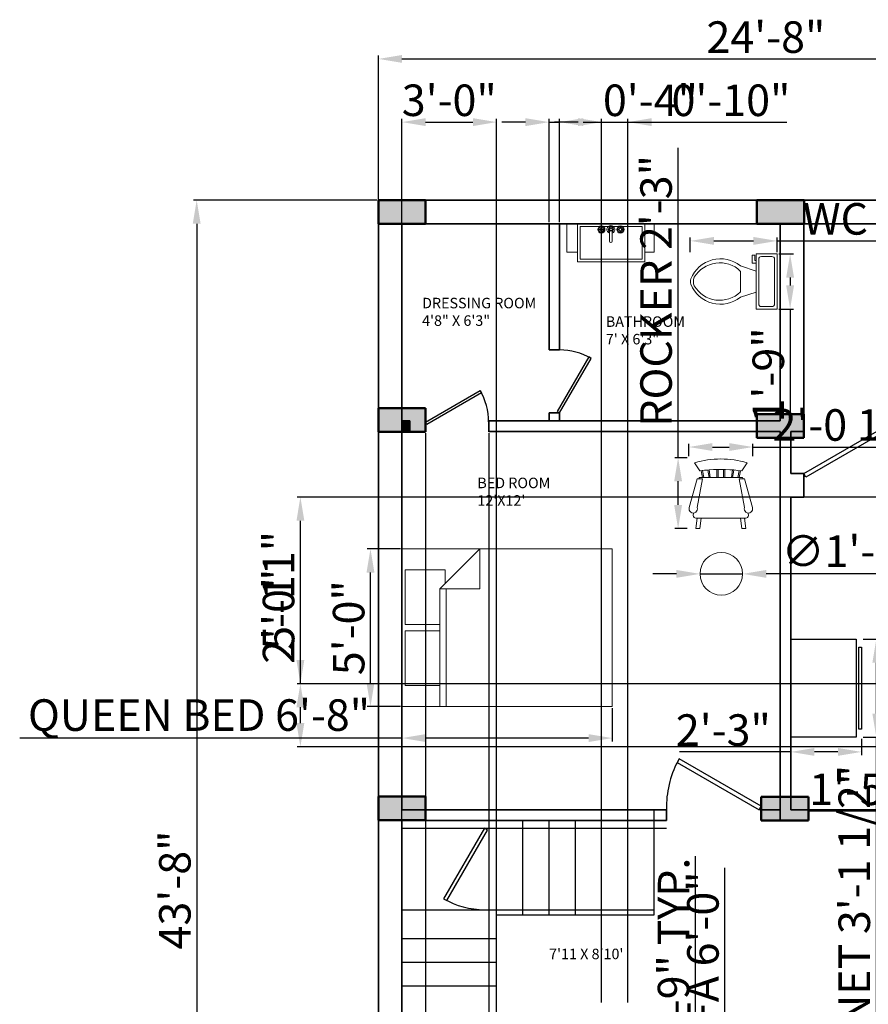
# Model space of a CAD drawing. Units: inches. Extents: x 1132 to 1713, y 3115 to 3781.
# Tile 2 of 4: x 1132 to 1455, y 3365 to 3740. Entities that reach past the tile are written whole.
import ezdxf

# ---------------------------------------------------------------- set-up
doc = ezdxf.new("R2010")
doc.units = ezdxf.units.IN
for name, color, linetype, lineweight in [('A-ANNO-DIMS', 2, 'Continuous', 18), ('A-AREA-IDEN', 7, 'Continuous', 18), ('A-COLS', 1, 'Continuous', 50), ('A-COLS-PATT', 252, 'Continuous', 13), ('A-DOOR', 3, 'Continuous', 25), ('A-FLOR-CASE', 30, 'Continuous', 25), ('A-FLOR-FIXT', 9, 'Continuous', 18), ('A-FLOR-STRS', 7, 'Continuous', 25), ('A-FURN', 8, 'Continuous', 18), ('A-WALL', 7, 'Continuous', 35)]:
    doc.layers.add(name, color=color, linetype=linetype, lineweight=lineweight)
doc.styles.get("Standard").update_dxf_attribs({"font": 'arial.ttf'})
doc.dimstyles.new('ISO-25', dxfattribs={"dimtxt": 12, "dimasz": 9, "dimexe": 1.25, "dimexo": 0.625, "dimtad": 1, "dimdec": 0, "dimrnd": 2, "dimlunit": 3, "dimtxsty": 'Standard', "dimcen": 2.5, "dimadec": 0, "dimazin": 0, "dimtfac": 1, "dimtdec": 0, "dimtmove": 0, "dimatfit": 3, "dimfxl": 1, "dimarcsym": 0})

# ---------------------------------------------------------------- blocks, each defined once
blk = doc.blocks.new('*U2')
for p, q in [((0, 0), (0, -6)), ((40, 0), (40, -6))]:
    blk.add_line(p, q)
blk.add_lwpolyline([(0, 0), (34.64, 20), (35.52, 18.48), (0.87, -1.52)], close=True)
blk.add_arc((0, 0), 40, 0, 30)
blk = doc.blocks.new('*U4')
for p, q in [((0, 0), (0, -6)), ((-40, 0), (-40, -6))]:
    blk.add_line(p, q)
blk.add_lwpolyline([(0, 0), (-34.64, 20), (-35.52, 18.48), (-0.88, -1.52)], close=True)
blk.add_arc((0, 0), 40, 150, 180)
blk = doc.blocks.new('*U3')
for p, q in [((0, 0), (0, 6)), ((40, 0), (40, 6))]:
    blk.add_line(p, q)
blk.add_lwpolyline([(0, 0), (34.64, -20), (35.52, -18.48), (0.87, 1.52)], close=True)
blk.add_arc((0, 0), 40, 330, 0)
blk = doc.blocks.new('*U5')
for p, q in [((0, 0), (0, -6)), ((-40, 0), (-40, -6))]:
    blk.add_line(p, q)
blk.add_lwpolyline([(0, 0), (-34.64, 20), (-35.52, 18.48), (-0.88, -1.52)], close=True)
blk.add_arc((0, 0), 40, 150, 180)
blk = doc.blocks.new('Toilet - top')
for p, q in [((9.5, -6), (9.5, -2)), ((-10, -8.5), (-8, -8.5)), ((-10, -9.5), (-10, -8.5)), ((-7, -9.5), (-10, -9.5)), ((-8, -8.5), (-8, -8)), ((-7, -8), (-7, -9.5)), ((-4, -8), (-6, -14)), ((4, -8), (6, -14)), ((4, -14), (-4, -14))]:
    blk.add_line(p, q)
blk.add_lwpolyline([(10.5, -8), (10.5, 0), (-10.5, 0), (-10.5, -8)], close=True)
for points in [[(-9.5, -2), (-9.5, -6)], [(8.5, -1), (-8.5, -1)], [(-8.5, -7), (8.5, -7)]]:
    blk.add_lwpolyline(points)
for centre, radius, start, end in [((-8.62, -1.88), 0.884, 81.8699, 188.1301), ((8.62, -1.88), 0.884, 351.8699, 98.1301), ((-8.62, -6.12), 0.884, 171.8699, 278.1301), ((8.62, -6.12), 0.884, 261.8699, 8.1301), ((3.52, -21.58), 12.17, 141.4691, 247.9714), ((4.2, -21.82), 11.33, 136.3677, 238.9468), ((-3.52, -21.58), 12.17, 292.0284, 38.5307), ((-4.2, -21.82), 11.33, 301.053, 43.6321), ((0, -27.88), 4, 245.7318, 294.2682), ((0, -29), 4, 254.8605, 285.1395)]:
    blk.add_arc(centre, radius, start, end)
blk = doc.blocks.new('Bed - Queen')
for p, q in [((0, -80.00003), (0, 0)), ((0, 0), (59.99999, 0)), ((59.99999, 0), (59.99999, -80.00003)), ((7.99999, -1.2), (28.79998, -1.2)), ((7.99999, -14.4), (7.99999, -1.2)), ((28.79998, -1.2), (28.79998, -14.4)), ((31.19999, -1.2), (51.99999, -1.2)), ((31.19999, -14.4), (31.19999, -1.2)), ((51.99999, -1.2), (51.99999, -16.4)), ((0, -14.4), (44.8, -14.4)), ((59.99999, -29.6), (44.8, -14.4)), ((44.8, -14.4), (44.8, -29.6)), ((44.8, -16.8), (0, -16.8)), ((51.99999, -16.4), (46.79936, -16.4)), ((44.8, -29.6), (59.99999, -29.6)), ((59.99999, -80.00003), (0, -80.00003))]:
    blk.add_line(p, q)
blk = doc.blocks.new('Chair - Rocking')
for p, q in [((-8, -4.5), (-10, -1.5)), ((8, -4.5), (10, -1.5)), ((-8.23428, -6.99939), (-8.3093, -7.47958)), ((-8.23041, -7), (8.23915, -7)), ((-7.5, -4.5), (-7, -7)), ((-6.5, -7), (-7.02225, -4.43)), ((-4.5, -7), (-4.96674, -4.19951)), ((-4, -7), (-4.40532, -4.16272)), ((-1.5, -4.05012), (-1.5, -7)), ((-1, -7), (-1, -4.05012)), ((1, -7), (1, -4.04655)), ((1.5, -4.05012), (1.5, -7)), ((4, -7), (4.40187, -4.18694)), ((4.5, -7), (4.96761, -4.19437)), ((6.5, -7), (7, -4.4057)), ((7.5, -4.5), (7, -7)), ((8.31071, -7.48854), (8.23449, -7.00073)), ((-9, -7.5), (-12, -18.49999)), ((-7, -7.5), (-9, -7.5)), ((-9, -18.49999), (-7, -7.5)), ((7, -7.5), (9, -7.5)), ((9, -18.49999), (7, -7.5)), ((9, -7.5), (12, -18.49999)), ((-10.36644, -20.64523), (-10.5, -21.49999)), ((10.5, -21.49999), (10.3575, -20.58798)), ((-9, -22.49999), (-9.5, -26.49999)), ((0, -22.49999), (-9.5, -22.49999)), ((-8, -26.49999), (-7.5, -22.49999)), ((0, -22.49999), (9.5, -22.49999)), ((8, -26.49999), (7.5, -22.49999)), ((9, -22.49999), (9.5, -26.49999)), ((-9.5, -26.49999), (-8, -26.49999)), ((9.5, -26.49999), (8, -26.49999))]:
    blk.add_line(p, q)
for centre, radius, start, end in [((0, -34.08333), 34.08333, 72.93847, 107.0615), ((0, -68.25004), 64.25, 93.92211, 97.15267), ((0, -68.25004), 64.25, 82.84733, 93.92211), ((-10.5, -18.99999), 1.58114, 161.5651, 18.43495), ((10.5, -18.99999), 1.58114, 161.5651, 18.43495), ((-9.5, -21.49999), 1, 180, 270), ((9.5, -21.49999), 1, 270, 0)]:
    blk.add_arc(centre, radius, start, end)
blk = doc.blocks.new('Wall Cabinet - 18 x 12 in side')
for points in [[(-12, -18), (-12, 0), (0, 0), (0, -18)], [(-13, -16.5), (-13, -1.5), (-12.5, -1.5), (-12.5, -16.5)]]:
    blk.add_lwpolyline(points, close=True)
blk = doc.blocks.new('*D18')
at = {"layer": 'A-ANNO-DIMS', "color": 0, "lineweight": -2, "transparency": 16777216}
for p, q in [((1267.53, 3670.88), (1197.76, 3670.88)), ((1199.01, 3661.88), (1199.01, 3154.88)), ((1267.53, 3145.88), (1197.76, 3145.88))]:
    blk.add_line(p, q, dxfattribs=at)
at = {"layer": 'A-ANNO-DIMS', "color": 0, "transparency": 16777216}
for points in [[(1197.51, 3661.88), (1200.51, 3661.88), (1199.01, 3670.88)], [(1197.51, 3154.88), (1200.51, 3154.88), (1199.01, 3145.88)]]:
    blk.add_solid(points, dxfattribs=at)
at = {"layer": 'Defpoints', "color": 0, "transparency": 16777216}
for p in [(1268.16, 3670.88), (1199.01, 3145.88), (1268.16, 3145.88)]:
    blk.add_point(p, dxfattribs=at)
at = {"layer": 'A-ANNO-DIMS', "color": 0, "transparency": 16777216, "insert": (1192.25, 3408.38), "char_height": 12, "attachment_point": 5, "rotation": 90}
blk.add_mtext('43\'-8"', dxfattribs=at)
blk = doc.blocks.new('*D19')
at = {"layer": 'A-ANNO-DIMS', "color": 0, "lineweight": -2, "transparency": 16777216}
for p, q in [((1268.16, 3667), (1268.16, 3725.86)), ((1277.16, 3724.61), (1554.22, 3724.61)), ((1563.22, 3671.51), (1563.22, 3725.86))]:
    blk.add_line(p, q, dxfattribs=at)
at = {"layer": 'A-ANNO-DIMS', "color": 0, "transparency": 16777216}
for points in [[(1277.16, 3726.11), (1277.16, 3723.11), (1268.16, 3724.61)], [(1554.22, 3726.11), (1554.22, 3723.11), (1563.22, 3724.61)]]:
    blk.add_solid(points, dxfattribs=at)
at = {"layer": 'Defpoints', "color": 0, "transparency": 16777216}
for p in [(1563.22, 3724.61), (1563.22, 3670.89), (1268.16, 3666.38)]:
    blk.add_point(p, dxfattribs=at)
at = {"layer": 'A-ANNO-DIMS', "color": 0, "transparency": 16777216, "insert": (1415.69, 3731.36), "char_height": 12, "attachment_point": 5}
blk.add_mtext('24\'-8"', dxfattribs=at)
blk = doc.blocks.new('Faucet - Bathroom top')
for p, q in [((-4.107, 0.125), (-4.375, 0.125)), ((-3.75, 0.4788), (-3.75, 0.75)), ((-3.5, 0.482), (-3.5, 0.75)), ((-3.1461, 0.125), (-2.875, 0.125)), ((3.143, 0.125), (2.875, 0.125)), ((3.5, 0.4788), (3.5, 0.75)), ((3.75, 0.482), (3.75, 0.75)), ((4.1039, 0.125), (4.375, 0.125)), ((-4.1039, -0.125), (-4.375, -0.125)), ((-3.75, -0.4821), (-3.75, -0.75)), ((-3.5, -0.4789), (-3.5, -0.75)), ((-3.143, -0.125), (-2.875, -0.125)), ((-0.5, -0.8639), (-0.5, -4.5)), ((0.5, -4.5), (0.5, -0.8631)), ((3.1461, -0.125), (2.875, -0.125)), ((3.5, -0.4821), (3.5, -0.75)), ((3.75, -0.4789), (3.75, -0.75)), ((4.107, -0.125), (4.375, -0.125))]:
    blk.add_line(p, q)
for centre, radius in [((-3.625, 0), 1.375), ((-4.625, 0), 0.2795), ((-3.625, 0), 0.5), ((-3.625, 1), 0.2795), ((-2.625, 0), 0.2795), ((0, 0), 0.5), ((3.625, 0), 1.375), ((2.625, 0), 0.2795), ((3.625, 0), 0.5), ((3.625, 1), 0.2795), ((4.625, 0), 0.2795), ((-3.625, -1), 0.2795), ((3.625, -1), 0.2795)]:
    blk.add_circle(centre, radius)
for centre, radius, start, end in [((-3.625, 0), 1, 105.2407, 164.2093), ((-3.625, 0), 1, 16.44125, 74.07887), ((0, 0), 1.5, 289.6514, 250.3603), ((0, 0), 1, 300.3431, 239.7554), ((3.625, 0), 1, 106.12, 164.0884), ((3.625, 0), 1, 16.23422, 73.90469), ((-3.625, 0), 1, 196.2342, 253.9047), ((-3.625, 0), 1, 286.12, 344.0884), ((3.625, 0), 1, 196.4413, 254.0789), ((3.625, 0), 1, 285.2407, 344.2093), ((0, -4.5), 0.5, 180, 0)]:
    blk.add_arc(centre, radius, start, end)
blk = doc.blocks.new('LAVATORY-WALL-MOUNT')
for p, q in [((-16.8, 2.17), (-16.8, -8.61)), ((16.5, -8.61), (16.5, 2.17)), ((-16.8, -8.61), (-12.71, -8.61)), ((12.88, -8.61), (16.5, -8.61))]:
    blk.add_line(p, q)
for points in [[(-12.71, 2.17), (12.88, 2.17), (12.88, -12.27), (-12.71, -12.27)], [(-11.71, 1.17), (11.88, 1.17), (11.88, -11.27), (-11.71, -11.27)]]:
    blk.add_lwpolyline(points, close=True)
for radius in [0.667, 0.447]:
    blk.add_circle((0, 0), radius)
blk.add_blockref('Faucet - Bathroom top', (0, 0))
blk = doc.blocks.new('*D22')
at = {"layer": 'A-ANNO-DIMS', "color": 0, "lineweight": -2, "transparency": 16777216}
for p, q in [((1382.27, 3572.88), (1382.27, 3690.79)), ((1385.69, 3572.88), (1381.02, 3572.88)), ((1382.27, 3554.88), (1382.27, 3563.88)), ((1385.69, 3545.88), (1381.02, 3545.88))]:
    blk.add_line(p, q, dxfattribs=at)
at = {"layer": 'A-ANNO-DIMS', "color": 0, "transparency": 16777216}
for points in [[(1380.77, 3563.88), (1383.77, 3563.88), (1382.27, 3572.88)], [(1380.77, 3554.88), (1383.77, 3554.88), (1382.27, 3545.88)]]:
    blk.add_solid(points, dxfattribs=at)
at = {"layer": 'Defpoints', "color": 0, "transparency": 16777216}
for p in [(1382.27, 3572.88), (1386.32, 3572.88), (1386.32, 3545.88)]:
    blk.add_point(p, dxfattribs=at)
at = {"layer": 'A-ANNO-DIMS', "color": 0, "transparency": 16777216, "insert": (1375.43, 3636.33), "char_height": 12, "attachment_point": 5, "rotation": 90}
blk.add_mtext('ROCKER 2\'-3"', dxfattribs=at)
blk = doc.blocks.new('*D23')
at = {"layer": 'A-ANNO-DIMS', "color": 0, "lineweight": -2, "transparency": 16777216}
for p, q in [((1386.32, 3573.51), (1386.32, 3578.18)), ((1410.75, 3573.51), (1410.75, 3578.18)), ((1395.32, 3576.93), (1401.75, 3576.93)), ((1410.75, 3576.93), (1481.07, 3576.93))]:
    blk.add_line(p, q, dxfattribs=at)
at = {"layer": 'A-ANNO-DIMS', "color": 0, "transparency": 16777216}
for points in [[(1395.32, 3578.43), (1395.32, 3575.43), (1386.32, 3576.93)], [(1401.75, 3578.43), (1401.75, 3575.43), (1410.75, 3576.93)]]:
    blk.add_solid(points, dxfattribs=at)
at = {"layer": 'Defpoints', "color": 0, "transparency": 16777216}
for p in [(1410.75, 3576.93), (1386.32, 3572.88), (1410.75, 3572.88)]:
    blk.add_point(p, dxfattribs=at)
at = {"layer": 'A-ANNO-DIMS', "color": 0, "transparency": 16777216, "insert": (1450.41, 3583.76), "char_height": 12, "attachment_point": 5}
blk.add_mtext('2\'-0 1/2"', dxfattribs=at)
blk = doc.blocks.new('*D25')
at = {"layer": 'A-ANNO-DIMS', "color": 0, "lineweight": -2, "transparency": 16777216}
for p, q in [((1523.43, 3440.62), (1523.43, 3437.14)), ((1540.66, 3440.62), (1540.66, 3437.14)), ((1514.43, 3438.39), (1432.17, 3438.39)), ((1540.66, 3438.39), (1523.43, 3438.39)), ((1549.66, 3438.39), (1558.66, 3438.39))]:
    blk.add_line(p, q, dxfattribs=at)
at = {"layer": 'A-ANNO-DIMS', "color": 0, "transparency": 16777216}
for points in [[(1514.43, 3439.89), (1514.43, 3436.89), (1523.43, 3438.39)], [(1549.66, 3439.89), (1549.66, 3436.89), (1540.66, 3438.39)]]:
    blk.add_solid(points, dxfattribs=at)
at = {"layer": 'Defpoints', "color": 0, "transparency": 16777216}
for p in [(1523.43, 3441.25), (1540.66, 3441.25), (1523.43, 3438.39)]:
    blk.add_point(p, dxfattribs=at)
at = {"layer": 'A-ANNO-DIMS', "color": 0, "transparency": 16777216, "insert": (1468.8, 3445.14), "char_height": 12, "attachment_point": 5}
blk.add_mtext('1\'-5" TYP.', dxfattribs=at)
blk = doc.blocks.new('*D27')
at = {"layer": 'A-ANNO-DIMS', "color": 0, "lineweight": -2, "transparency": 16777216}
for p, q in [((1388.83, 3337.88), (1388.83, 3421.27)), ((1384.06, 3328.88), (1390.08, 3328.88)), ((1388.83, 3319.88), (1388.83, 3328.88)), ((1384.06, 3319.88), (1390.08, 3319.88)), ((1388.83, 3310.88), (1388.83, 3301.88))]:
    blk.add_line(p, q, dxfattribs=at)
at = {"layer": 'A-ANNO-DIMS', "color": 0, "transparency": 16777216}
for points in [[(1387.33, 3337.88), (1390.33, 3337.88), (1388.83, 3328.88)], [(1387.33, 3310.88), (1390.33, 3310.88), (1388.83, 3319.88)]]:
    blk.add_solid(points, dxfattribs=at)
at = {"layer": 'Defpoints', "color": 0, "transparency": 16777216}
for p in [(1383.43, 3328.88), (1388.83, 3328.88), (1383.43, 3319.88)]:
    blk.add_point(p, dxfattribs=at)
at = {"layer": 'A-ANNO-DIMS', "color": 0, "transparency": 16777216, "insert": (1382.08, 3384.07), "char_height": 12, "attachment_point": 5, "rotation": 90}
blk.add_mtext('0\'-9" TYP.', dxfattribs=at)
blk = doc.blocks.new('*D32')
at = {"layer": 'A-ANNO-DIMS', "color": 0, "lineweight": -2, "transparency": 16777216}
for p, q in [((1400.1, 3324.4), (1400.1, 3416.8)), ((1410.25, 3324.4), (1398.85, 3324.4)), ((1400.1, 3261.57), (1400.1, 3315.4)), ((1410.25, 3252.57), (1398.85, 3252.57))]:
    blk.add_line(p, q, dxfattribs=at)
at = {"layer": 'A-ANNO-DIMS', "color": 0, "transparency": 16777216}
for points in [[(1398.6, 3315.4), (1401.6, 3315.4), (1400.1, 3324.4)], [(1398.6, 3261.57), (1401.6, 3261.57), (1400.1, 3252.57)]]:
    blk.add_solid(points, dxfattribs=at)
at = {"layer": 'Defpoints', "color": 0, "transparency": 16777216}
for p in [(1400.1, 3324.4), (1410.88, 3324.4), (1410.88, 3252.57)]:
    blk.add_point(p, dxfattribs=at)
at = {"layer": 'A-ANNO-DIMS', "color": 0, "transparency": 16777216, "insert": (1393.27, 3375.1), "char_height": 12, "attachment_point": 5, "rotation": 90}
blk.add_mtext('SOFA 6\'-0"', dxfattribs=at)
blk = doc.blocks.new('*D36')
at = {"layer": 'A-ANNO-DIMS', "color": 0, "lineweight": -2, "transparency": 16777216}
for p, q in [((1386.9, 3651.03), (1386.9, 3656.61)), ((1395.9, 3655.36), (1410.95, 3655.36)), ((1419.95, 3651.03), (1419.95, 3656.61)), ((1419.95, 3655.36), (1495.17, 3655.36))]:
    blk.add_line(p, q, dxfattribs=at)
at = {"layer": 'A-ANNO-DIMS', "color": 0, "transparency": 16777216}
for points in [[(1395.9, 3656.86), (1395.9, 3653.86), (1386.9, 3655.36)], [(1410.95, 3656.86), (1410.95, 3653.86), (1419.95, 3655.36)]]:
    blk.add_solid(points, dxfattribs=at)
at = {"layer": 'Defpoints', "color": 0, "transparency": 16777216}
for p in [(1419.95, 3655.36), (1386.9, 3650.4), (1419.95, 3650.4)]:
    blk.add_point(p, dxfattribs=at)
at = {"layer": 'A-ANNO-DIMS', "color": 0, "transparency": 16777216, "insert": (1462.06, 3662.19), "char_height": 12, "attachment_point": 5}
blk.add_mtext('WC 2\'-9"', dxfattribs=at)
blk = doc.blocks.new('*D37')
at = {"layer": 'A-ANNO-DIMS', "color": 0, "lineweight": -2, "transparency": 16777216}
for p, q in [((1420.57, 3650.4), (1426.15, 3650.4)), ((1424.9, 3641.4), (1424.9, 3638.4)), ((1420.57, 3629.4), (1426.15, 3629.4)), ((1424.9, 3629.4), (1424.9, 3588.38))]:
    blk.add_line(p, q, dxfattribs=at)
at = {"layer": 'A-ANNO-DIMS', "color": 0, "transparency": 16777216}
for points in [[(1423.4, 3641.4), (1426.4, 3641.4), (1424.9, 3650.4)], [(1423.4, 3638.4), (1426.4, 3638.4), (1424.9, 3629.4)]]:
    blk.add_solid(points, dxfattribs=at)
at = {"layer": 'Defpoints', "color": 0, "transparency": 16777216}
for p in [(1419.95, 3650.4), (1419.95, 3629.4), (1424.9, 3629.4)]:
    blk.add_point(p, dxfattribs=at)
at = {"layer": 'A-ANNO-DIMS', "color": 0, "transparency": 16777216, "insert": (1418.15, 3604.39), "char_height": 12, "attachment_point": 5, "rotation": 90}
blk.add_mtext('1\'-9"', dxfattribs=at)
blk = doc.blocks.new('*D38')
at = {"layer": 'A-ANNO-DIMS', "color": 0, "lineweight": -2, "transparency": 16777216}
for p, q in [((1277.16, 3477.56), (1277.16, 3464.93)), ((1357.16, 3477.56), (1357.16, 3464.93)), ((1277.16, 3466.18), (1131.64, 3466.18)), ((1348.16, 3466.18), (1286.16, 3466.18))]:
    blk.add_line(p, q, dxfattribs=at)
at = {"layer": 'A-ANNO-DIMS', "color": 0, "transparency": 16777216}
for points in [[(1286.16, 3467.68), (1286.16, 3464.68), (1277.16, 3466.18)], [(1348.16, 3467.68), (1348.16, 3464.68), (1357.16, 3466.18)]]:
    blk.add_solid(points, dxfattribs=at)
at = {"layer": 'Defpoints', "color": 0, "transparency": 16777216}
for p in [(1277.16, 3478.18), (1357.16, 3478.18), (1277.16, 3466.18)]:
    blk.add_point(p, dxfattribs=at)
at = {"layer": 'A-ANNO-DIMS', "color": 0, "transparency": 16777216, "insert": (1199.9, 3473.38), "char_height": 12, "attachment_point": 5}
blk.add_mtext('QUEEN BED 6\'-8"', dxfattribs=at)
blk = doc.blocks.new('*D39')
at = {"layer": 'A-ANNO-DIMS', "color": 0, "lineweight": -2, "transparency": 16777216}
for p, q in [((1276.53, 3538.18), (1263.91, 3538.18)), ((1265.16, 3487.18), (1265.16, 3529.18)), ((1276.53, 3478.18), (1263.91, 3478.18))]:
    blk.add_line(p, q, dxfattribs=at)
at = {"layer": 'A-ANNO-DIMS', "color": 0, "transparency": 16777216}
for points in [[(1263.66, 3529.18), (1266.66, 3529.18), (1265.16, 3538.18)], [(1263.66, 3487.18), (1266.66, 3487.18), (1265.16, 3478.18)]]:
    blk.add_solid(points, dxfattribs=at)
at = {"layer": 'Defpoints', "color": 0, "transparency": 16777216}
for p in [(1265.16, 3538.18), (1277.16, 3538.18), (1277.16, 3478.18)]:
    blk.add_point(p, dxfattribs=at)
at = {"layer": 'A-ANNO-DIMS', "color": 0, "transparency": 16777216, "insert": (1258.41, 3508.18), "char_height": 12, "attachment_point": 5, "rotation": 90}
blk.add_mtext('5\'-0"', dxfattribs=at)
blk = doc.blocks.new('*D40')
at = {"layer": 'A-ANNO-DIMS', "color": 0, "lineweight": -2, "transparency": 16777216}
for p, q in [((1452.73, 3503.82), (1458.96, 3503.82)), ((1457.71, 3494.82), (1457.71, 3475.51)), ((1452.73, 3466.51), (1458.96, 3466.51)), ((1457.71, 3466.51), (1457.71, 3319.22))]:
    blk.add_line(p, q, dxfattribs=at)
at = {"layer": 'A-ANNO-DIMS', "color": 0, "transparency": 16777216}
for points in [[(1456.21, 3494.82), (1459.21, 3494.82), (1457.71, 3503.82)], [(1456.21, 3475.51), (1459.21, 3475.51), (1457.71, 3466.51)]]:
    blk.add_solid(points, dxfattribs=at)
at = {"layer": 'Defpoints', "color": 0, "transparency": 16777216}
for p in [(1452.11, 3503.82), (1452.11, 3466.51), (1457.71, 3466.51)]:
    blk.add_point(p, dxfattribs=at)
at = {"layer": 'A-ANNO-DIMS', "color": 0, "transparency": 16777216, "insert": (1450.87, 3388.36), "char_height": 12, "attachment_point": 5, "rotation": 90}
blk.add_mtext('CABINET 3\'-1 1/2"', dxfattribs=at)
blk = doc.blocks.new('*D41')
at = {"layer": 'A-ANNO-DIMS', "color": 0, "lineweight": -2, "transparency": 16777216}
for p, q in [((1425.16, 3465.88), (1425.16, 3459.66)), ((1452.11, 3465.88), (1452.11, 3459.66)), ((1425.16, 3460.91), (1382.81, 3460.91)), ((1443.11, 3460.91), (1434.16, 3460.91))]:
    blk.add_line(p, q, dxfattribs=at)
at = {"layer": 'A-ANNO-DIMS', "color": 0, "transparency": 16777216}
for points in [[(1434.16, 3462.41), (1434.16, 3459.41), (1425.16, 3460.91)], [(1443.11, 3462.41), (1443.11, 3459.41), (1452.11, 3460.91)]]:
    blk.add_solid(points, dxfattribs=at)
at = {"layer": 'Defpoints', "color": 0, "transparency": 16777216}
for p in [(1425.16, 3466.51), (1452.11, 3466.51), (1425.16, 3460.91)]:
    blk.add_point(p, dxfattribs=at)
at = {"layer": 'A-ANNO-DIMS', "color": 0, "transparency": 16777216, "insert": (1399.48, 3467.67), "char_height": 12, "attachment_point": 5}
blk.add_mtext('2\'-3"', dxfattribs=at)
blk = doc.blocks.new('*D46')
at = {"layer": 'A-ANNO-DIMS', "color": 0, "lineweight": -2, "transparency": 16777216}
for p, q in [((1277.16, 3363.5), (1277.16, 3701.81)), ((1313.16, 3365.5), (1313.16, 3701.81)), ((1286.16, 3700.56), (1304.16, 3700.56))]:
    blk.add_line(p, q, dxfattribs=at)
at = {"layer": 'A-ANNO-DIMS', "color": 0, "transparency": 16777216}
for points in [[(1286.16, 3702.06), (1286.16, 3699.06), (1277.16, 3700.56)], [(1304.16, 3702.06), (1304.16, 3699.06), (1313.16, 3700.56)]]:
    blk.add_solid(points, dxfattribs=at)
at = {"layer": 'Defpoints', "color": 0, "transparency": 16777216}
for p in [(1313.16, 3700.56), (1313.16, 3364.88), (1277.16, 3362.88)]:
    blk.add_point(p, dxfattribs=at)
at = {"layer": 'A-ANNO-DIMS', "color": 0, "transparency": 16777216, "insert": (1295.16, 3707.32), "char_height": 12, "attachment_point": 5}
blk.add_mtext('3\'-0"', dxfattribs=at)
blk = doc.blocks.new('*D47')
at = {"layer": 'A-ANNO-DIMS', "color": 0, "lineweight": -2, "transparency": 16777216}
for p, q in [((1353.16, 3365.5), (1353.16, 3701.81)), ((1363.16, 3365.5), (1363.16, 3701.81)), ((1344.16, 3700.56), (1335.16, 3700.56)), ((1353.16, 3700.56), (1363.16, 3700.56)), ((1372.16, 3700.56), (1423.63, 3700.56))]:
    blk.add_line(p, q, dxfattribs=at)
at = {"layer": 'A-ANNO-DIMS', "color": 0, "transparency": 16777216}
for points in [[(1344.16, 3702.06), (1344.16, 3699.06), (1353.16, 3700.56)], [(1372.16, 3702.06), (1372.16, 3699.06), (1363.16, 3700.56)]]:
    blk.add_solid(points, dxfattribs=at)
at = {"layer": 'Defpoints', "color": 0, "transparency": 16777216}
for p in [(1363.16, 3700.56), (1353.16, 3364.88), (1363.16, 3364.88)]:
    blk.add_point(p, dxfattribs=at)
at = {"layer": 'A-ANNO-DIMS', "color": 0, "transparency": 16777216, "insert": (1402.4, 3707.31), "char_height": 12, "attachment_point": 5}
blk.add_mtext('0\'-10"', dxfattribs=at)
blk = doc.blocks.new('*D53')
at = {"layer": 'A-ANNO-DIMS', "color": 0, "lineweight": -2, "transparency": 16777216}
for p, q in [((1286.16, 3582.14), (1286.16, 3114.9)), ((1310.16, 3582.25), (1310.16, 3114.9)), ((1295.16, 3116.15), (1301.16, 3116.15)), ((1310.16, 3116.15), (1352.51, 3116.15))]:
    blk.add_line(p, q, dxfattribs=at)
at = {"layer": 'A-ANNO-DIMS', "color": 0, "transparency": 16777216}
for points in [[(1295.16, 3117.65), (1295.16, 3114.65), (1286.16, 3116.15)], [(1301.16, 3117.65), (1301.16, 3114.65), (1310.16, 3116.15)]]:
    blk.add_solid(points, dxfattribs=at)
at = {"layer": 'Defpoints', "color": 0, "transparency": 16777216}
for p in [(1286.16, 3582.77), (1310.16, 3582.88), (1310.16, 3116.15)]:
    blk.add_point(p, dxfattribs=at)
at = {"layer": 'A-ANNO-DIMS', "color": 0, "transparency": 16777216, "insert": (1335.84, 3122.9), "char_height": 12, "attachment_point": 5}
blk.add_mtext('2\'-0"', dxfattribs=at)
blk = doc.blocks.new('*D54')
at = {"layer": 'A-ANNO-DIMS', "color": 0, "lineweight": -2, "transparency": 16777216}
for p, q in [((1333.16, 3662.5), (1333.16, 3701.81)), ((1337.16, 3662.5), (1337.16, 3701.81)), ((1324.16, 3700.56), (1315.16, 3700.56)), ((1333.16, 3700.56), (1337.16, 3700.56)), ((1346.16, 3700.56), (1388.31, 3700.56))]:
    blk.add_line(p, q, dxfattribs=at)
at = {"layer": 'A-ANNO-DIMS', "color": 0, "transparency": 16777216}
for points in [[(1324.16, 3702.06), (1324.16, 3699.06), (1333.16, 3700.56)], [(1346.16, 3702.06), (1346.16, 3699.06), (1337.16, 3700.56)]]:
    blk.add_solid(points, dxfattribs=at)
at = {"layer": 'Defpoints', "color": 0, "transparency": 16777216}
for p in [(1337.16, 3700.56), (1333.16, 3661.88), (1337.16, 3661.88)]:
    blk.add_point(p, dxfattribs=at)
at = {"layer": 'A-ANNO-DIMS', "color": 0, "transparency": 16777216, "insert": (1371.73, 3707.31), "char_height": 12, "attachment_point": 5}
blk.add_mtext('0\'-4"', dxfattribs=at)
blk = doc.blocks.new('*D56')
at = {"layer": 'A-ANNO-DIMS', "color": 0, "lineweight": -2, "transparency": 16777216}
for p, q in [((1238.49, 3486.88), (1238.49, 3529.23)), ((1493.53, 3486.88), (1237.24, 3486.88)), ((1238.49, 3471.88), (1238.49, 3477.88)), ((1493.53, 3462.88), (1237.24, 3462.88))]:
    blk.add_line(p, q, dxfattribs=at)
at = {"layer": 'A-ANNO-DIMS', "color": 0, "transparency": 16777216}
for points in [[(1236.99, 3477.88), (1239.99, 3477.88), (1238.49, 3486.88)], [(1236.99, 3471.88), (1239.99, 3471.88), (1238.49, 3462.88)]]:
    blk.add_solid(points, dxfattribs=at)
at = {"layer": 'Defpoints', "color": 0, "transparency": 16777216}
for p in [(1238.49, 3486.88), (1494.16, 3486.88), (1494.16, 3462.88)]:
    blk.add_point(p, dxfattribs=at)
at = {"layer": 'A-ANNO-DIMS', "color": 0, "transparency": 16777216, "insert": (1231.73, 3512.55), "char_height": 12, "attachment_point": 5, "rotation": 90}
blk.add_mtext('2\'-0"', dxfattribs=at)
blk = doc.blocks.new('*D57')
at = {"layer": 'A-ANNO-DIMS', "color": 0, "lineweight": -2, "transparency": 16777216}
for p, q in [((1517.53, 3557.88), (1237.24, 3557.88)), ((1238.49, 3495.88), (1238.49, 3548.88)), ((1517.53, 3486.88), (1237.24, 3486.88))]:
    blk.add_line(p, q, dxfattribs=at)
at = {"layer": 'A-ANNO-DIMS', "color": 0, "transparency": 16777216}
for points in [[(1236.99, 3548.88), (1239.99, 3548.88), (1238.49, 3557.88)], [(1236.99, 3495.88), (1239.99, 3495.88), (1238.49, 3486.88)]]:
    blk.add_solid(points, dxfattribs=at)
at = {"layer": 'Defpoints', "color": 0, "transparency": 16777216}
for p in [(1238.49, 3557.88), (1518.16, 3557.88), (1518.16, 3486.88)]:
    blk.add_point(p, dxfattribs=at)
at = {"layer": 'A-ANNO-DIMS', "color": 0, "transparency": 16777216, "insert": (1231.73, 3522.38), "char_height": 12, "attachment_point": 5, "rotation": 90}
blk.add_mtext('5\'-11"', dxfattribs=at)
blk = doc.blocks.new('*D59')
at = {"layer": 'A-ANNO-DIMS', "color": 0, "lineweight": -2, "transparency": 16777216}
for p, q in [((1381.6, 3528.66), (1372.6, 3528.66)), ((1390.6, 3528.66), (1406.81, 3528.66)), ((1471.02, 3528.66), (1415.81, 3528.66))]:
    blk.add_line(p, q, dxfattribs=at)
at = {"layer": 'A-ANNO-DIMS', "color": 0, "transparency": 16777216}
for points in [[(1381.6, 3530.16), (1381.6, 3527.16), (1390.6, 3528.66)], [(1415.81, 3530.16), (1415.81, 3527.16), (1406.81, 3528.66)]]:
    blk.add_solid(points, dxfattribs=at)
at = {"layer": 'Defpoints', "color": 0, "transparency": 16777216}
for p in [(1390.6, 3528.66), (1406.81, 3528.66)]:
    blk.add_point(p, dxfattribs=at)
at = {"layer": 'A-ANNO-DIMS', "color": 0, "transparency": 16777216, "insert": (1447.92, 3535.75), "char_height": 12, "attachment_point": 5, "rotation": 0.002}
blk.add_mtext('∅1\'-4"', dxfattribs=at)

msp = doc.modelspace()

# ---------------------------------------------------------------- hatches: boundary and pattern name
at = {"layer": 'A-COLS-PATT'}
h = msp.add_hatch(color=256, dxfattribs=at)
h.dxf.hatch_style = 1
h.paths.add_polyline_path([(1286.16, 3661.88), (1286.16, 3670.88), (1268.16, 3670.88), (1268.16, 3661.88)])
h = msp.add_hatch(color=256, dxfattribs=at)
h.dxf.hatch_style = 1
h.paths.add_polyline_path([(1430.21, 3661.88), (1430.21, 3670.88), (1412.21, 3670.88), (1412.21, 3661.88)])
h = msp.add_hatch(color=256, dxfattribs=at)
h.dxf.hatch_style = 1
h.paths.add_polyline_path([(1277.16, 3591.77), (1268.16, 3591.77), (1268.16, 3582.77), (1277.16, 3582.77), (1277.16, 3582.88), (1277.16, 3586.88)])
h = msp.add_hatch(color=256, dxfattribs=at)
h.dxf.hatch_style = 1
h.paths.add_polyline_path([(1280.16, 3586.88), (1280.16, 3582.88), (1277.16, 3582.88), (1277.16, 3582.77), (1286.16, 3582.77), (1286.16, 3591.77), (1277.16, 3591.77), (1277.16, 3586.88)])
h = msp.add_hatch(color=256, dxfattribs=at)
h.dxf.hatch_style = 1
h.paths.add_polyline_path([(1412.17, 3586.88), (1412.17, 3582.88), (1421.16, 3582.88), (1421.16, 3580.44), (1425.16, 3580.44), (1425.16, 3582.88), (1430.16, 3582.88), (1430.16, 3589.44), (1421.16, 3589.44), (1421.16, 3586.88)])
h = msp.add_hatch(color=256, dxfattribs=at)
h.dxf.hatch_style = 1
h.paths.add_polyline_path([(1421.16, 3582.88), (1421.16, 3580.44), (1425.16, 3580.44), (1425.16, 3582.88), (1430.16, 3582.88), (1430.16, 3589.44), (1421.16, 3589.44), (1421.16, 3586.88), (1412.17, 3586.88), (1412.17, 3582.88)])
h = msp.add_hatch(color=256, dxfattribs=at)
h.dxf.hatch_style = 1
h.paths.add_polyline_path([(1412.17, 3589.44), (1412.17, 3586.88), (1421.16, 3586.88), (1421.16, 3589.44)])
h = msp.add_hatch(color=256, dxfattribs=at)
h.dxf.hatch_style = 1
h.paths.add_polyline_path([(1277.16, 3582.88), (1280.16, 3582.88), (1280.16, 3586.88), (1277.16, 3586.88)])
h = msp.add_hatch(color=256, dxfattribs=at)
h.dxf.hatch_style = 1
h.paths.add_polyline_path([(1421.16, 3580.44), (1421.16, 3582.88), (1412.17, 3582.88), (1412.17, 3580.44)])
h = msp.add_hatch(color=256, dxfattribs=at)
h.dxf.hatch_style = 1
h.paths.add_polyline_path([(1425.16, 3582.88), (1425.16, 3580.44), (1430.17, 3580.44), (1430.17, 3582.88)])
h = msp.add_hatch(color=256, dxfattribs=at)
h.dxf.hatch_style = 1
h.paths.add_polyline_path([(1268.16, 3443.91), (1268.16, 3434.91), (1286.16, 3434.91), (1286.16, 3438.88), (1277.16, 3438.88), (1277.16, 3443.91)])
h = msp.add_hatch(color=256, dxfattribs=at)
h.dxf.hatch_style = 1
h.paths.add_polyline_path([(1277.16, 3443.91), (1277.16, 3438.88), (1286.16, 3438.88), (1286.16, 3443.91)])
h = msp.add_hatch(color=256, dxfattribs=at)
h.dxf.hatch_style = 1
h.paths.add_polyline_path([(1421.16, 3438.88), (1421.16, 3443.88), (1413.86, 3443.88), (1413.86, 3438.88)])
h = msp.add_hatch(color=256, dxfattribs=at)
h.dxf.hatch_style = 1
h.paths.add_polyline_path([(1425.16, 3438.88), (1425.16, 3443.88), (1421.16, 3443.88), (1421.16, 3434.88), (1431.86, 3434.88), (1431.86, 3438.88)])
h = msp.add_hatch(color=256, dxfattribs=at)
h.dxf.hatch_style = 1
h.paths.add_polyline_path([(1431.86, 3438.88), (1431.86, 3443.88), (1425.16, 3443.88), (1425.16, 3438.88)])
h = msp.add_hatch(color=256, dxfattribs=at)
h.dxf.hatch_style = 1
h.paths.add_polyline_path([(1413.86, 3438.88), (1413.86, 3434.88), (1421.16, 3434.88), (1421.16, 3438.88)])

# ---------------------------------------------------------------- linework, layer by layer
at = {"layer": 'A-COLS'}
for p, q in [((1268.16, 3670.88), (1268.16, 3661.88)), ((1286.16, 3670.88), (1268.16, 3670.88)), ((1268.16, 3670.88), (1268.16, 3661.88)), ((1286.16, 3661.88), (1286.16, 3670.88)), ((1286.16, 3661.88), (1286.16, 3670.88)), ((1430.21, 3670.88), (1412.21, 3670.88)), ((1412.21, 3670.88), (1412.21, 3661.88)), ((1430.21, 3661.88), (1430.21, 3670.88)), ((1268.16, 3661.88), (1286.16, 3661.88)), ((1268.16, 3661.88), (1286.16, 3661.88)), ((1412.21, 3661.88), (1430.21, 3661.88)), ((1286.16, 3591.77), (1268.16, 3591.77)), ((1268.16, 3591.77), (1268.16, 3582.77)), ((1286.16, 3582.77), (1286.16, 3591.77)), ((1430.17, 3589.44), (1412.17, 3589.44)), ((1412.17, 3589.44), (1412.17, 3580.44)), ((1430.17, 3580.44), (1430.17, 3589.44)), ((1268.16, 3582.77), (1286.16, 3582.77)), ((1412.17, 3580.44), (1430.17, 3580.44)), ((1286.16, 3443.91), (1268.16, 3443.91)), ((1268.16, 3443.91), (1268.16, 3434.91)), ((1286.16, 3434.91), (1286.16, 3443.91)), ((1431.86, 3443.88), (1413.86, 3443.88)), ((1413.86, 3443.88), (1413.86, 3434.88)), ((1431.86, 3434.88), (1431.86, 3443.88)), ((1268.16, 3434.91), (1286.16, 3434.91)), ((1413.86, 3434.88), (1431.86, 3434.88))]:
    msp.add_line(p, q, dxfattribs=at)
at = {"layer": 'A-FLOR-STRS'}
for p, q in [((1373.16, 3398.88), (1373.16, 3438.88)), ((1313.16, 3328.88), (1313.16, 3434.88)), ((1313.16, 3431.88), (1313.16, 3434.88)), ((1323.16, 3398.88), (1323.16, 3434.88)), ((1333.16, 3398.88), (1333.16, 3434.88)), ((1343.16, 3398.88), (1343.16, 3434.88)), ((1353.16, 3398.88), (1353.16, 3434.88)), ((1363.16, 3398.88), (1363.16, 3434.88)), ((1277.16, 3431.88), (1377.86, 3431.88)), ((1277.16, 3400.88), (1373.16, 3400.88)), ((1313.16, 3398.88), (1373.16, 3398.88)), ((1277.16, 3389.88), (1313.16, 3389.88)), ((1277.16, 3380.88), (1313.16, 3380.88)), ((1277.16, 3371.88), (1313.16, 3371.88))]:
    msp.add_line(p, q, dxfattribs=at)
at = {"layer": 'A-FURN'}
msp.add_circle((1398.71, 3528.66), 8.11, dxfattribs=at)
at = {"layer": 'A-WALL'}
for p, q in [((1277.16, 3661.88), (1421.16, 3661.88)), ((1277.16, 3582.88), (1277.16, 3661.88)), ((1333.16, 3613.88), (1333.16, 3661.88)), ((1337.16, 3613.88), (1337.16, 3661.88)), ((1421.16, 3586.88), (1421.16, 3661.88)), ((1421.16, 3586.88), (1421.16, 3661.88)), ((1430.16, 3582.88), (1430.16, 3661.88)), ((1430.16, 3661.88), (1554.16, 3661.88)), ((1333.16, 3613.88), (1337.16, 3613.88)), ((1333.16, 3586.88), (1333.16, 3589.88)), ((1333.16, 3589.88), (1337.16, 3589.88)), ((1337.16, 3586.88), (1337.16, 3589.88)), ((1277.16, 3586.88), (1280.16, 3586.88)), ((1277.16, 3582.88), (1277.16, 3586.88)), ((1280.16, 3582.88), (1280.16, 3586.88)), ((1310.16, 3586.88), (1421.16, 3586.88)), ((1310.16, 3582.77), (1310.16, 3586.88)), ((1333.16, 3586.88), (1337.16, 3586.88)), ((1277.16, 3582.88), (1280.16, 3582.88)), ((1277.16, 3438.88), (1277.16, 3582.88)), ((1310.16, 3582.88), (1421.16, 3582.88)), ((1421.16, 3434.88), (1421.16, 3582.88)), ((1425.16, 3566.88), (1425.16, 3582.88)), ((1425.16, 3582.88), (1430.16, 3582.88)), ((1421.16, 3557.88), (1421.16, 3566.88)), ((1425.16, 3566.88), (1430.16, 3566.88)), ((1430.16, 3557.88), (1430.16, 3566.88)), ((1425.16, 3557.88), (1430.16, 3557.88)), ((1425.16, 3438.88), (1425.16, 3557.88)), ((1277.16, 3438.88), (1377.86, 3438.88)), ((1377.86, 3438.88), (1377.86, 3434.88)), ((1413.86, 3438.88), (1421.16, 3438.88)), ((1425.16, 3438.88), (1554.16, 3438.88)), ((1277.16, 3434.88), (1377.86, 3434.88)), ((1277.16, 3328.88), (1277.16, 3434.88))]:
    msp.add_line(p, q, dxfattribs=at)
msp.add_lwpolyline([(1268.16, 3670.88), (1563.16, 3670.88), (1563.16, 3145.88), (1268.16, 3145.88)], close=True, dxfattribs=at)

# ---------------------------------------------------------------- block references
at = {"layer": 'A-DOOR'}
for name, p, xscale, yscale, zscale, rotation in [('*U3', (1337.16, 3589.88), 0.6000000000000005, 0.6000000000000005, 0.6000000000000005, 89.99999999999991), ('*U2', (1286.14, 3586.37), 0.6000058349880895, 0.6000058349880895, 0.6000058349880895, 0.25268544818529), ('*U5', (1308.51, 3431.88), 0.7750000000000008, 0.7750000000000008, 0.7750000000000008, 89.99999999999991)]:
    msp.add_blockref(name, p, dxfattribs=dict(at, xscale=xscale, yscale=yscale, zscale=zscale, rotation=rotation))
at = {"layer": 'A-DOOR', "xscale": 0.9, "yscale": 0.9, "zscale": 0.9}
for name, p in [('*U2', (1430.16, 3566.88)), ('*U4', (1413.86, 3440.28))]:
    msp.add_blockref(name, p, dxfattribs=at)
at = {"layer": 'A-FLOR-CASE', "xscale": 2.073042315474223, "yscale": 2.073042315474223, "zscale": 2.073042315474223, "rotation": 180}
msp.add_blockref('Wall Cabinet - 18 x 12 in side', (1425.16, 3466.51), dxfattribs=at)
at = {"layer": 'A-FLOR-FIXT'}
msp.add_blockref('LAVATORY-WALL-MOUNT', (1356.67, 3659.71), dxfattribs=at)
at = {"layer": 'A-FLOR-FIXT', "rotation": 270}
msp.add_blockref('Toilet - top', (1419.95, 3639.9), dxfattribs=at)
at = {"layer": 'A-FURN'}
msp.add_blockref('Chair - Rocking', (1398.53, 3572.38), dxfattribs=at)
at = {"layer": 'A-FURN', "rotation": 90}
msp.add_blockref('Bed - Queen', (1277.16, 3478.18), dxfattribs=at)

# ---------------------------------------------------------------- texts
at = {"layer": 'A-AREA-IDEN', "char_height": 4, "attachment_point": 1}
for s, insert in [('{\\fArial|b1|i0|c0|p34;DRESSING ROOM\\P4\'8" X 6\'3"}', (1284.81, 3633.71)), ('{\\fArial|b1|i0|c0|p34;BATHROOM\\P7\' X 6\'3"}', (1354.75, 3626.65)), ("{\\fArial|b1|i0|c0|p34;BED ROOM \\P12'X12'}", (1305.85, 3565.27)), ("{\\fArial|b1|i0|c0|p34;7'11 X 8'10'}", (1333.16, 3386.04))]:
    msp.add_mtext_dynamic_manual_height_columns(s, width=83.7568, gutter_width=12.5, heights=[54.87], dxfattribs=dict(at, insert=insert))

# ---------------------------------------------------------------- dimensions: what is measured, and where the dimension line sits
at = {"layer": 'A-ANNO-DIMS'}
for base, p1, p2, override, picture, middle in [((1563.22, 3724.61), (1268.16, 3666.38), (1563.22, 3670.89), {"dimclrd": 0, "dimclre": 0, "dimclrt": 0}, '*D19', (1415.69, 3731.36)), ((1313.16, 3700.56), (1277.16, 3362.88), (1313.16, 3364.88), {"dimdec": 1, "dimlfac": 1, "dimrnd": 0, "dimzin": 1, "dimdsep": 46, "dimlunit": 4, "dimfrac": 2}, '*D46', (1295.16, 3707.32)), ((1337.16, 3700.56), (1333.16, 3661.88), (1337.16, 3661.88), {"dimdec": 1, "dimlfac": 1, "dimrnd": 0, "dimzin": 1, "dimdsep": 46, "dimlunit": 4, "dimfrac": 2}, '*D54', (1371.73, 3707.31)), ((1363.16, 3700.56), (1353.16, 3364.88), (1363.16, 3364.88), {"dimdec": 1, "dimlfac": 1, "dimrnd": 0, "dimzin": 1, "dimdsep": 46, "dimlunit": 4, "dimfrac": 2}, '*D47', (1402.4, 3707.31)), ((1410.75, 3576.93), (1386.32, 3572.88), (1410.75, 3572.88), {"dimdec": 1, "dimlfac": 1, "dimrnd": 0, "dimzin": 1, "dimdsep": 46, "dimlunit": 4, "dimfrac": 2}, '*D23', (1450.41, 3583.76)), ((1310.16, 3116.15), (1286.16, 3582.77), (1310.16, 3582.88), {"dimdec": 1, "dimlfac": 1, "dimrnd": 0, "dimzin": 1, "dimdsep": 46, "dimlunit": 4, "dimfrac": 2}, '*D53', (1335.84, 3122.9))]:
    dim = msp.add_linear_dim(base=base, p1=p1, p2=p2, dimstyle='ISO-25', override=override, dxfattribs=at)
    dim.commit()
    dim.dimension.update_dxf_attribs({"geometry": picture, "text_midpoint": middle})
for base, p1, p2, angle, text, picture, middle in [((1382.27, 3572.88), (1386.32, 3545.88), (1386.32, 3572.88), 90, 'ROCKER <>', '*D22', (1375.43, 3636.33)), ((1457.71, 3466.51), (1452.11, 3503.82), (1452.11, 3466.51), 270, 'CABINET <>', '*D40', (1450.87, 3388.36)), ((1277.16, 3466.18), (1357.16, 3478.18), (1277.16, 3478.18), 180, 'QUEEN BED <>', '*D38', (1199.9, 3473.38)), ((1523.43, 3438.39), (1540.66, 3441.25), (1523.43, 3441.25), 180, '<> TYP.', '*D25', (1468.8, 3445.14)), ((1388.83, 3328.88), (1383.43, 3319.88), (1383.43, 3328.88), 90, '<> TYP.', '*D27', (1382.08, 3384.07)), ((1400.1, 3324.4), (1410.88, 3252.57), (1410.88, 3324.4), 90, 'SOFA <>', '*D32', (1393.27, 3375.1))]:
    dim = msp.add_linear_dim(base=base, p1=p1, p2=p2, angle=angle, text=text, dimstyle='ISO-25', override={"dimdec": 1, "dimlfac": 1, "dimrnd": 0, "dimzin": 1, "dimdsep": 46, "dimlunit": 4, "dimfrac": 2}, dxfattribs=at)
    dim.commit()
    dim.dimension.update_dxf_attribs({"geometry": picture, "text_midpoint": middle})
dim = msp.add_linear_dim(base=(1419.9459, 3655.3614), p1=(1386.8997, 3650.4044), p2=(1419.9459, 3650.4044), text='WC <>', dimstyle='ISO-25', override={"dimdec": 1, "dimlfac": 1, "dimrnd": 0, "dimzin": 1, "dimdsep": 46, "dimlunit": 4, "dimfrac": 2}, dxfattribs=at)
dim.commit()
dim.dimension.update_dxf_attribs({"geometry": '*D36', "text_midpoint": (1462.0593, 3662.191)})
for base, p1, p2, angle, override, picture, middle in [((1199.01, 3145.88), (1268.16, 3670.88), (1268.16, 3145.88), 90, {"dimclrd": 0, "dimclre": 0, "dimclrt": 0}, '*D18', (1192.25, 3408.38)), ((1424.9, 3629.4), (1419.95, 3650.4), (1419.95, 3629.4), 270, {"dimdec": 1, "dimlfac": 1, "dimrnd": 0, "dimzin": 1, "dimdsep": 46, "dimlunit": 4, "dimfrac": 2}, '*D37', (1418.15, 3604.39)), ((1238.49, 3557.88), (1518.16, 3486.88), (1518.16, 3557.88), 90, {"dimdec": 1, "dimlfac": 1, "dimrnd": 0, "dimzin": 1, "dimdsep": 46, "dimlunit": 4, "dimfrac": 2}, '*D57', (1231.73, 3522.38)), ((1265.16, 3538.18), (1277.16, 3478.18), (1277.16, 3538.18), 90, {"dimdec": 1, "dimlfac": 1, "dimrnd": 0, "dimzin": 1, "dimdsep": 46, "dimlunit": 4, "dimfrac": 2}, '*D39', (1258.41, 3508.18)), ((1238.49, 3486.88), (1494.16, 3462.88), (1494.16, 3486.88), 90, {"dimdec": 1, "dimlfac": 1, "dimrnd": 0, "dimzin": 1, "dimdsep": 46, "dimlunit": 4, "dimfrac": 2}, '*D56', (1231.73, 3512.55)), ((1425.1599, 3460.9095), (1452.1095, 3466.5067), (1425.1599, 3466.5067), 180, {"dimdec": 1, "dimlfac": 1, "dimrnd": 0, "dimzin": 1, "dimdsep": 46, "dimlunit": 4, "dimfrac": 2}, '*D41', (1399.4831, 3467.6654))]:
    dim = msp.add_linear_dim(base=base, p1=p1, p2=p2, angle=angle, dimstyle='ISO-25', override=override, dxfattribs=at)
    dim.commit()
    dim.dimension.update_dxf_attribs({"geometry": picture, "text_midpoint": middle})
dim = msp.add_diameter_dim_2p(p1=(1390.6, 3528.66), p2=(1406.81, 3528.66), dimstyle='ISO-25', override={"dimdec": 1, "dimlfac": 1, "dimrnd": 0, "dimzin": 1, "dimdsep": 46, "dimlunit": 4, "dimfrac": 2}, dxfattribs=at)
dim.commit()
dim.dimension.update_dxf_attribs({"geometry": '*D59', "text_midpoint": (1447.92, 3528.66), "dimtype": 163})

doc.saveas('drawing.dxf')
